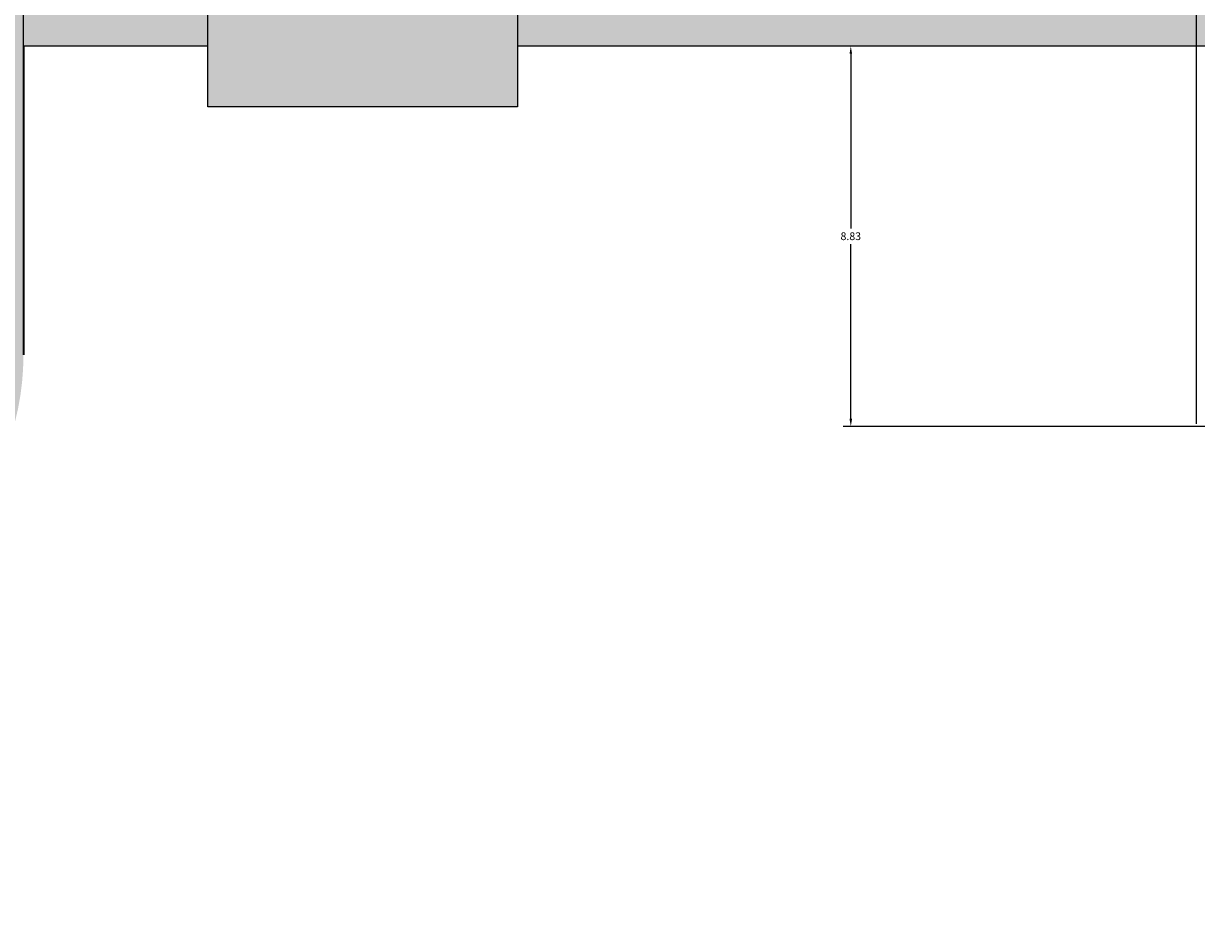
# Model space of a CAD drawing. Units: millimetres. Extents: x -11 to 280, y -4 to 208.
# Tile 22 of 55: x 91 to 119, y 85 to 106. Entities that reach past the tile are written whole.
import ezdxf

# ---------------------------------------------------------------- set-up
doc = ezdxf.new("R2010")
doc.units = ezdxf.units.MM
for name, color, linetype, lineweight in [('M-DIMS', 2, 'Continuous', 18), ('M-HYDR-EQPM', 7, 'Continuous', 35), ('M-HYDR-PRES', 7, 'Continuous', 25), ('M-HYDR-SUCT', 7, 'Continuous', 25), ('M-HYDR-VALV', 7, 'Continuous', 25)]:
    doc.layers.add(name, color=color, linetype=linetype, lineweight=lineweight)
doc.layers.add('M-HYDR-PRES-PATT', color=240, linetype='Continuous', lineweight=13, true_color=0xed1f24)
doc.layers.add('M-HYDR-SUCT-PATT', color=221, linetype='Continuous', lineweight=13, true_color=0xff7fdf)
doc.styles.get("Standard").update_dxf_attribs({"font": 'arial.ttf'})
doc.dimstyles.get("Standard").update_dxf_attribs({"dimtxt": 0.18, "dimasz": 0.18, "dimexe": 0.18, "dimexo": 0.0625, "dimgap": 0.09, "dimtad": 0, "dimtih": 1, "dimtoh": 1, "dimdec": 4, "dimzin": 0, "dimdsep": 46, "dimtxsty": 'Standard', "dimcen": 0.09, "dimadec": 0, "dimazin": 0, "dimtfac": 1, "dimtdec": 4, "dimtofl": 0, "dimtmove": 0, "dimatfit": 3, "dimfxl": 1, "dimtolj": 1, "dimtzin": 0, "dimarcsym": 0})

# ---------------------------------------------------------------- blocks, each defined once
blk = doc.blocks.new('*D5')
at = {"layer": 'Defpoints', "color": 0, "transparency": 16777216}
for p in [(24.759, 192.645), (-10.087, 11.435), (261.686, 11.435)]:
    blk.add_point(p, dxfattribs=at)
at = {"layer": 'M-DIMS', "color": 0, "lineweight": -2, "transparency": 16777216}
for p, q in [((24.696, 192.645), (-10.267, 192.645)), ((-10.087, 192.465), (-10.087, 102.222)), ((-10.087, 11.615), (-10.087, 101.858)), ((261.624, 11.435), (-10.267, 11.435))]:
    blk.add_line(p, q, dxfattribs=at)
at = {"layer": 'M-DIMS', "color": 0, "transparency": 16777216}
for points in [[(-10.117, 192.465), (-10.057, 192.465), (-10.087, 192.645)], [(-10.117, 11.615), (-10.057, 11.615), (-10.087, 11.435)]]:
    blk.add_solid(points, dxfattribs=at)
at = {"layer": 'M-DIMS', "color": 0, "transparency": 16777216, "insert": (-10.087, 102.04), "char_height": 0.18, "attachment_point": 5}
blk.add_mtext('\\A1;181.2', dxfattribs=at)
blk = doc.blocks.new('*D11')
at = {"layer": 'Defpoints', "color": 0, "transparency": 16777216}
for p in [(118.514, 207.495), (91.3, 98.149), (118.514, 96.485)]:
    blk.add_point(p, dxfattribs=at)
at = {"layer": 'M-DIMS', "color": 0, "lineweight": -2, "transparency": 16777216}
for p, q in [((91.3, 98.212), (91.3, 207.675)), ((118.514, 96.547), (118.514, 207.675)), ((91.48, 207.495), (104.442, 207.495)), ((118.334, 207.495), (105.372, 207.495))]:
    blk.add_line(p, q, dxfattribs=at)
at = {"layer": 'M-DIMS', "color": 0, "transparency": 16777216}
for points in [[(91.48, 207.525), (91.48, 207.465), (91.3, 207.495)], [(118.334, 207.525), (118.334, 207.465), (118.514, 207.495)]]:
    blk.add_solid(points, dxfattribs=at)
at = {"layer": 'M-DIMS', "color": 0, "transparency": 16777216, "insert": (104.907, 207.495), "char_height": 0.18, "attachment_point": 5}
blk.add_mtext('\\A1;27.214', dxfattribs=at)
blk = doc.blocks.new('*D12')
at = {"layer": 'Defpoints', "color": 0, "transparency": 16777216}
for p in [(173.804, 207.495), (118.514, 96.485), (173.804, 89.387)]:
    blk.add_point(p, dxfattribs=at)
at = {"layer": 'M-DIMS', "color": 0, "lineweight": -2, "transparency": 16777216}
for p, q in [((118.514, 96.547), (118.514, 207.675)), ((173.804, 89.45), (173.804, 207.675)), ((118.694, 207.495), (145.765, 207.495)), ((173.624, 207.495), (146.553, 207.495))]:
    blk.add_line(p, q, dxfattribs=at)
at = {"layer": 'M-DIMS', "color": 0, "transparency": 16777216}
for points in [[(118.694, 207.525), (118.694, 207.465), (118.514, 207.495)], [(173.624, 207.525), (173.624, 207.465), (173.804, 207.495)]]:
    blk.add_solid(points, dxfattribs=at)
at = {"layer": 'M-DIMS', "color": 0, "transparency": 16777216, "insert": (146.159, 207.495), "char_height": 0.18, "attachment_point": 5}
blk.add_mtext('\\A1;55.29', dxfattribs=at)
blk = doc.blocks.new('*D16')
at = {"layer": 'Defpoints', "color": 0, "transparency": 16777216}
for p in [(110.493, 105.314), (125.343, 105.314), (125.343, 96.485)]:
    blk.add_point(p, dxfattribs=at)
at = {"layer": 'M-DIMS', "color": 0, "lineweight": -2, "transparency": 16777216}
for p, q in [((125.281, 105.314), (110.313, 105.314)), ((110.493, 105.134), (110.493, 101.081)), ((110.493, 96.665), (110.493, 100.718)), ((125.281, 96.485), (110.313, 96.485))]:
    blk.add_line(p, q, dxfattribs=at)
at = {"layer": 'M-DIMS', "color": 0, "transparency": 16777216}
for points in [[(110.463, 105.134), (110.523, 105.134), (110.493, 105.314)], [(110.463, 96.665), (110.523, 96.665), (110.493, 96.485)]]:
    blk.add_solid(points, dxfattribs=at)
at = {"layer": 'M-DIMS', "color": 0, "transparency": 16777216, "insert": (110.493, 100.9), "char_height": 0.18, "attachment_point": 5}
blk.add_mtext('\\A1;8.83', dxfattribs=at)

msp = doc.modelspace()

# ---------------------------------------------------------------- hatches: boundary and pattern name
at = {"layer": 'M-HYDR-PRES-PATT'}
h = msp.add_hatch(color=256, dxfattribs=at)
h.set_gradient(color1=(237, 31, 36), color2=(237, 31, 36), tint=1)
h.paths.add_polyline_path([(232.2, 133.1228), (228.7, 133.1228), (228.7, 108.8141), (102.7646, 108.8141), (102.7646, 105.3141), (232.2, 105.3141)])
h.paths.add_polyline_path([(128.8433, 105.3141), (125.3433, 105.3141), (125.3433, 91.7099, 1), (128.8433, 91.7099)])
h.paths.add_polyline_path([(229.1617, 78.7098), (196.7745, 78.7098, -0.4142136), (191.7745, 83.7098), (191.7745, 105.3141), (188.2745, 105.3141), (188.2745, 80.2098, 0.4142136), (193.2745, 75.2098), (225.6617, 75.2098), (225.6617, 43.5991), (229.1617, 43.5991)])
h.paths.add_polyline_path([(102.7646, 110.3704), (95.5776, 110.3704), (95.5776, 103.9022), (102.7646, 103.9022)])
h.paths.add_polyline_path([(100.7059, 107.2502), (99.1711, 106.3641), (99.1711, 106.8641), (97.1711, 106.8641), (97.1711, 107.6363), (99.1711, 107.6363), (99.1711, 108.1363)], flags=16)
h.paths.add_polyline_path([(234.6119, 138.4081), (226.5106, 138.4081), (226.5106, 133.1228), (234.6119, 133.1228)])
h.paths.add_polyline_path([(231.1963, 135.7055), (230.2965, 134.1786), (229.4241, 135.7213), (229.9241, 135.7168), (229.9418, 137.7167), (230.7141, 137.7099), (230.6963, 135.71)], flags=16)
at = {"layer": 'M-HYDR-SUCT-PATT'}
h = msp.add_hatch(color=256, dxfattribs=at)
h.set_gradient(color1=(255, 127, 223), color2=(255, 127, 223), tint=1, name='INVCYLINDER')
h.paths.add_polyline_path([(91.3629, 155.4768), (91.3629, 132.4768), (58.3629, 132.4768), (58.3629, 153.9768), (54.8629, 153.9768), (54.8629, 128.9768), (94.8629, 128.9768), (94.8629, 151.9768), (205.5315, 151.9768), (205.5315, 155.4768)])
h.paths.add_polyline_path([(91.3, 114.9452, 1), (78.8273, 114.9452), (78.8273, 108.8141), (42.6453, 108.8141), (42.6453, 153.9768), (39.1453, 153.9768), (39.1453, 105.3141), (78.8273, 105.3141), (78.8273, 98.1491, 1), (91.3, 98.1491), (91.3, 105.3141), (95.5776, 105.3141), (95.5776, 108.8141), (91.3, 108.8141)])
h.paths.add_polyline_path([(228.7, 138.4081), (232.2, 138.4081), (232.2, 144.6609), (228.7, 144.6609)])
h.paths.add_polyline_path([(253.1005, 151.9768, 1), (253.1005, 155.4768), (252.6001, 155.4768), (253.5249, 153.991, -0.1401047), (253.6005, 153.7268, -0.7542249), (252.676, 153.4626), (251.4221, 155.4768), (236.9353, 155.4768), (236.9353, 151.9768)])
h.paths.add_polyline_path([(30.8182, 40.7626), (30.8182, 36.7626), (60.8182, 36.7626), (60.8182, 40.7626)])

# ---------------------------------------------------------------- linework, layer by layer
at = {"layer": 'M-HYDR-EQPM'}
msp.add_lwpolyline([(91.3, 105.3141), (91.3, 98.1491)], dxfattribs=at)
at = {"layer": 'M-HYDR-PRES'}
msp.add_lwpolyline([(232.2, 133.1228), (232.2, 105.3141), (102.7646, 105.3141)], dxfattribs=at)
at = {"layer": 'M-HYDR-SUCT'}
msp.add_lwpolyline([(95.5776, 105.3141), (91.3, 105.3141)], dxfattribs=at)
at = {"layer": 'M-HYDR-VALV'}
msp.add_lwpolyline([(95.5776, 110.3704), (102.7646, 110.3704), (102.7646, 103.9022), (95.5776, 103.9022)], close=True, dxfattribs=at)

# ---------------------------------------------------------------- dimensions: what is measured, and where the dimension line sits
at = {"layer": 'M-DIMS'}
for base, p1, p2, override, picture, middle in [((118.5137, 207.495), (91.3, 98.1491), (118.5137, 96.4849), {"dimdec": 3, "dimlfac": 1, "dimrnd": 0, "dimzin": 0, "dimdsep": 46, "dimlunit": 2}, '*D11', (104.9068, 207.495)), ((173.8038, 207.495), (118.5137, 96.4849), (173.8038, 89.3873), {"dimdec": 2, "dimlfac": 1, "dimrnd": 0, "dimzin": 0, "dimdsep": 46, "dimlunit": 2}, '*D12', (146.1587, 207.495))]:
    dim = msp.add_linear_dim(base=base, p1=p1, p2=p2, dimstyle='Standard', override=override, dxfattribs=at)
    dim.commit()
    dim.dimension.update_dxf_attribs({"geometry": picture, "text_midpoint": middle})
for base, p1, p2, override, picture, middle in [((-10.0865, 11.4346), (24.7588, 192.645), (261.6863, 11.4346), {"dimdec": 1, "dimlfac": 1, "dimrnd": 0, "dimzin": 0, "dimdsep": 46, "dimlunit": 2}, '*D5', (-10.0865, 102.0398)), ((110.4933, 105.3141), (125.3433, 96.4849), (125.3433, 105.3141), {"dimdec": 2, "dimlfac": 1, "dimrnd": 0, "dimzin": 0, "dimdsep": 46, "dimlunit": 2}, '*D16', (110.4933, 100.8995))]:
    dim = msp.add_linear_dim(base=base, p1=p1, p2=p2, angle=90, dimstyle='Standard', override=override, dxfattribs=at)
    dim.commit()
    dim.dimension.update_dxf_attribs({"geometry": picture, "text_midpoint": middle})

doc.saveas('drawing.dxf')
